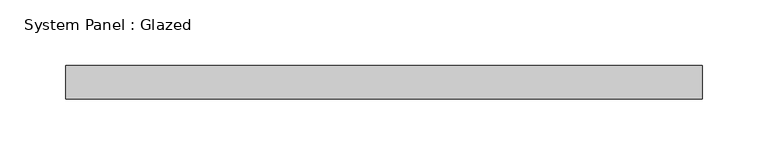
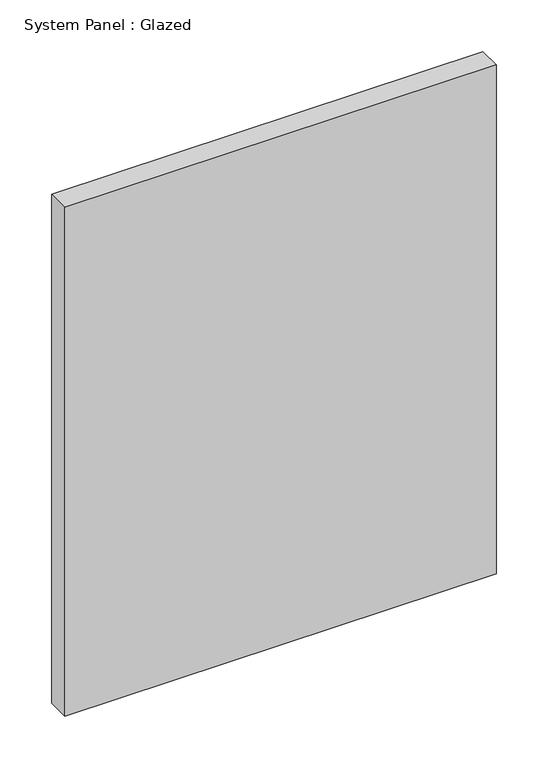
"""IFC4 building model written with IfcOpenShell, lengths in millimetres: plate geometry, System Panel : Glazed."""

from ifc_helpers import new_model, si_unit, origin, origin_with_axes, place, context, project, spatial, polyline, outline, extrude, source, transform, mapped, element, save


def system_panel_glazed_9cf13bc3(model_context):
    return source(origin(), model_context, "Body", "SweptSolid", [
        extrude(outline(polyline([(241.3, 19.05), (-241.3, 19.05), (-241.3, 44.45), (241.3, 44.45), (241.3, 19.05)])), origin_with_axes(), (0.0, 0.0, 1.0), 601.9642589),
    ])


if __name__ == "__main__":
    model = new_model("IFC4")
    model_context = context("Model", 3, world=origin())
    ifc_project = project(units=[si_unit("LENGTHUNIT", "METRE", prefix="MILLI")], contexts=[model_context])
    site = spatial("IfcSite", under=ifc_project)
    building = spatial("IfcBuilding", under=site)
    placement = place(None, origin())
    system_panel_glazed_shape = system_panel_glazed_9cf13bc3(model_context)
    element("IfcPlate", 1, ObjectType="System Panel : Glazed", at=placement, inside=building, context=model_context, shape_type="MappedRepresentation", body=[
        mapped(system_panel_glazed_shape, transform((0.0, 0.0, 0.0), x_axis=(1.0, 0.0, 0.0), y_axis=(0.0, 1.0, 0.0), z_axis=(0.0, 0.0, 1.0))),
    ])
    save(model, "model.ifc")

# Revit data of these elements
# Type "System Panel : Glazed"
#   Construction Type Id = "GSP4R"
#   Analytic Construction = "1/8 in Pilkington single glazing"
#   Visual Light Transmittance = 0.9
#   Solar Heat Gain Coefficient = 0.86
#   Heat Transfer Coefficient (U) = 1.18115 BTU/(h·ft²·°F)
#   Define Thermal Properties by = 1
# Element 1 (IfcPlate, "System Panel : Glazed")
#   Materials on its faces: "Glass"
# Materials
#   "Glass": class "Glass", colour RGB 0 128 192, transparency 0.75, Description = "Soda Lime Glass", Cost = 0
